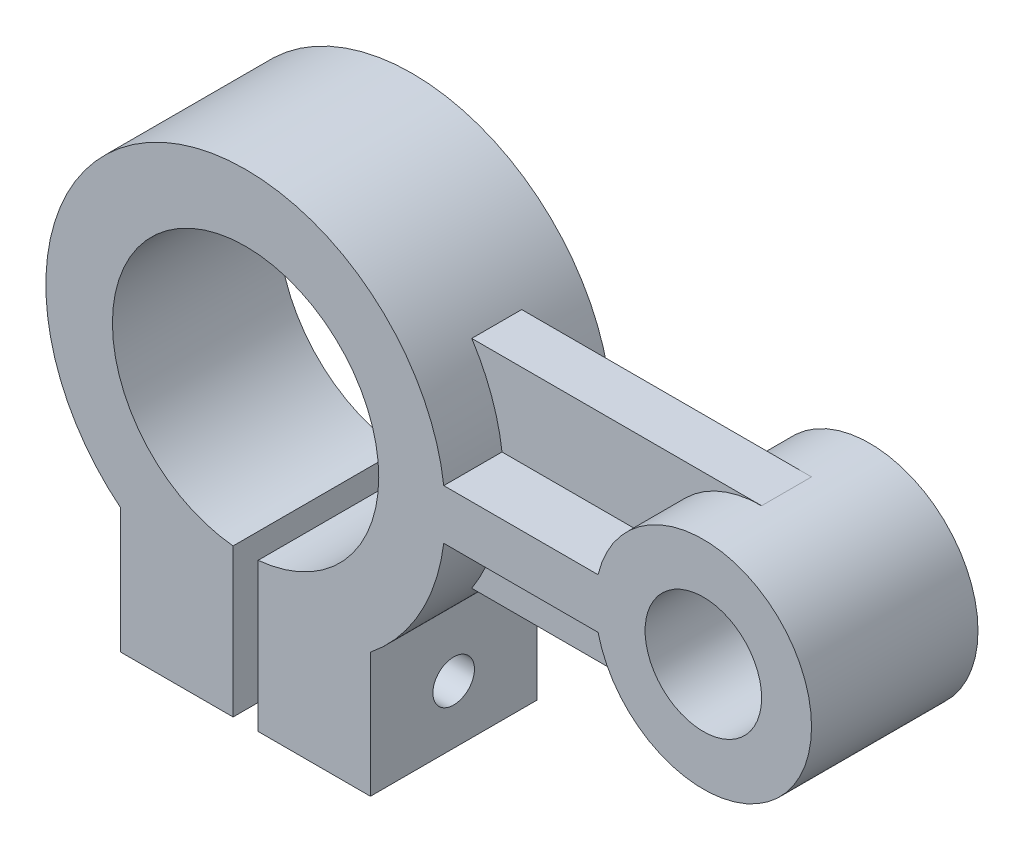
ISO-10303-21;
HEADER;
FILE_DESCRIPTION(('STEP AP214'),'2;1');
FILE_NAME('part.step','',(''),(''),'','','');
FILE_SCHEMA(('AUTOMOTIVE_DESIGN { 1 0 10303 214 1 1 1 1 }'));
ENDSEC;
DATA;
#1=APPLICATION_CONTEXT('core data for automotive mechanical design processes');
#2=APPLICATION_PROTOCOL_DEFINITION('international standard','automotive_design',2000,#1);
#3=PRODUCT_CONTEXT('',#1,'mechanical');
#4=PRODUCT('Part','Part','',(#3));
#5=PRODUCT_RELATED_PRODUCT_CATEGORY('part','',(#4));
#6=PRODUCT_DEFINITION_FORMATION('','',#4);
#7=PRODUCT_DEFINITION_CONTEXT('part definition',#1,'design');
#8=PRODUCT_DEFINITION('design','',#6,#7);
#9=PRODUCT_DEFINITION_SHAPE('','',#8);
#10=(LENGTH_UNIT() NAMED_UNIT(*) SI_UNIT(.MILLI.,.METRE.));
#11=(NAMED_UNIT(*) PLANE_ANGLE_UNIT() SI_UNIT($,.RADIAN.));
#12=(NAMED_UNIT(*) SI_UNIT($,.STERADIAN.) SOLID_ANGLE_UNIT());
#13=UNCERTAINTY_MEASURE_WITH_UNIT(LENGTH_MEASURE(1.E-05),#10,'distance_accuracy_value','');
#14=(GEOMETRIC_REPRESENTATION_CONTEXT(3) GLOBAL_UNCERTAINTY_ASSIGNED_CONTEXT((#13)) GLOBAL_UNIT_ASSIGNED_CONTEXT((#10,
#11,#12)) REPRESENTATION_CONTEXT('',''));
#15=CARTESIAN_POINT('',(0.,0.,0.));
#16=DIRECTION('',(0.,0.,1.));
#17=DIRECTION('',(1.,0.,0.));
#18=AXIS2_PLACEMENT_3D('',#15,#16,#17);
#19=CARTESIAN_POINT('',(30.,-67.4699879903904,-20.));
#20=DIRECTION('',(0.,-1.,0.));
#21=DIRECTION('',(1.,0.,0.));
#22=AXIS2_PLACEMENT_3D('',#19,#20,#21);
#23=PLANE('',#22);
#24=DIRECTION('',(0.,0.,1.));
#25=VECTOR('',#24,1.);
#26=CARTESIAN_POINT('',(-3.,-67.4699879903904,-20.));
#27=LINE('',#26,#25);
#28=CARTESIAN_POINT('',(-3.,-67.4699879903904,-20.));
#29=VERTEX_POINT('',#28);
#30=CARTESIAN_POINT('',(-3.,-67.4699879903904,20.));
#31=VERTEX_POINT('',#30);
#32=EDGE_CURVE('E179',#29,#31,#27,.T.);
#33=ORIENTED_EDGE('',*,*,#32,.T.);
#34=DIRECTION('',(1.,0.,0.));
#35=VECTOR('',#34,1.);
#36=CARTESIAN_POINT('',(30.,-67.4699879903904,20.));
#37=LINE('',#36,#35);
#38=CARTESIAN_POINT('',(-30.,-67.4699879903904,20.));
#39=VERTEX_POINT('',#38);
#40=EDGE_CURVE('E217',#39,#31,#37,.T.);
#41=ORIENTED_EDGE('',*,*,#40,.F.);
#42=DIRECTION('',(0.,0.,1.));
#43=VECTOR('',#42,1.);
#44=CARTESIAN_POINT('',(-30.,-67.4699879903904,-20.));
#45=LINE('',#44,#43);
#46=CARTESIAN_POINT('',(-30.,-67.4699879903904,-20.));
#47=VERTEX_POINT('',#46);
#48=EDGE_CURVE('E202',#47,#39,#45,.T.);
#49=ORIENTED_EDGE('',*,*,#48,.F.);
#50=DIRECTION('',(1.,0.,0.));
#51=VECTOR('',#50,1.);
#52=CARTESIAN_POINT('',(30.,-67.4699879903904,-20.));
#53=LINE('',#52,#51);
#54=EDGE_CURVE('E197',#47,#29,#53,.T.);
#55=ORIENTED_EDGE('',*,*,#54,.T.);
#56=EDGE_LOOP('',(#33,#41,#49,#55));
#57=FACE_BOUND('',#56,.T.);
#58=ADVANCED_FACE('F44',(#57),#23,.T.);
#59=CARTESIAN_POINT('',(0.,0.,20.));
#60=DIRECTION('',(0.,0.,-1.));
#61=DIRECTION('',(-1.,0.,0.));
#62=AXIS2_PLACEMENT_3D('',#59,#60,#61);
#63=CYLINDRICAL_SURFACE('',#62,48.);
#64=CARTESIAN_POINT('',(0.,0.,20.));
#65=DIRECTION('',(0.,0.,1.));
#66=DIRECTION('',(1.,0.,0.));
#67=AXIS2_PLACEMENT_3D('',#64,#65,#66);
#68=CIRCLE('',#67,48.);
#69=CARTESIAN_POINT('',(30.,-37.4699879903904,20.));
#70=VERTEX_POINT('',#69);
#71=CARTESIAN_POINT('',(47.6235235991626,-6.,20.));
#72=VERTEX_POINT('',#71);
#73=EDGE_CURVE('E324',#70,#72,#68,.T.);
#74=ORIENTED_EDGE('',*,*,#73,.F.);
#75=DIRECTION('',(0.,0.,1.));
#76=VECTOR('',#75,1.);
#77=CARTESIAN_POINT('',(30.,-37.4699879903904,-20.));
#78=LINE('',#77,#76);
#79=CARTESIAN_POINT('',(30.,-37.4699879903904,-20.));
#80=VERTEX_POINT('',#79);
#81=EDGE_CURVE('E221',#80,#70,#78,.T.);
#82=ORIENTED_EDGE('',*,*,#81,.F.);
#83=CARTESIAN_POINT('',(0.,0.,-20.));
#84=DIRECTION('',(0.,0.,1.));
#85=DIRECTION('',(1.,0.,0.));
#86=AXIS2_PLACEMENT_3D('',#83,#84,#85);
#87=CIRCLE('',#86,48.);
#88=CARTESIAN_POINT('',(47.6235235991626,-6.,-20.));
#89=VERTEX_POINT('',#88);
#90=EDGE_CURVE('E320',#80,#89,#87,.T.);
#91=ORIENTED_EDGE('',*,*,#90,.T.);
#92=DIRECTION('',(0.,0.,-1.));
#93=VECTOR('',#92,1.);
#94=CARTESIAN_POINT('',(47.6235235991626,-6.,20.));
#95=LINE('',#94,#93);
#96=CARTESIAN_POINT('',(47.6235235991626,-6.,-6.));
#97=VERTEX_POINT('',#96);
#98=EDGE_CURVE('E309',#89,#97,#95,.F.);
#99=ORIENTED_EDGE('',*,*,#98,.T.);
#100=CARTESIAN_POINT('',(0.,0.,-6.));
#101=DIRECTION('',(0.,0.,-1.));
#102=DIRECTION('',(-1.,0.,0.));
#103=AXIS2_PLACEMENT_3D('',#100,#101,#102);
#104=CIRCLE('',#103,48.);
#105=CARTESIAN_POINT('',(40.348482003664,-26.,-6.));
#106=VERTEX_POINT('',#105);
#107=EDGE_CURVE('E259',#97,#106,#104,.T.);
#108=ORIENTED_EDGE('',*,*,#107,.T.);
#109=DIRECTION('',(0.,0.,-1.));
#110=VECTOR('',#109,1.);
#111=CARTESIAN_POINT('',(40.348482003664,-26.,20.));
#112=LINE('',#111,#110);
#113=CARTESIAN_POINT('',(40.348482003664,-26.,6.));
#114=VERTEX_POINT('',#113);
#115=EDGE_CURVE('E261',#114,#106,#112,.T.);
#116=ORIENTED_EDGE('',*,*,#115,.F.);
#117=CARTESIAN_POINT('',(0.,0.,6.));
#118=DIRECTION('',(0.,0.,-1.));
#119=DIRECTION('',(-1.,0.,0.));
#120=AXIS2_PLACEMENT_3D('',#117,#118,#119);
#121=CIRCLE('',#120,48.);
#122=CARTESIAN_POINT('',(47.6235235991626,-6.,6.));
#123=VERTEX_POINT('',#122);
#124=EDGE_CURVE('E260',#123,#114,#121,.T.);
#125=ORIENTED_EDGE('',*,*,#124,.F.);
#126=EDGE_CURVE('E306',#123,#72,#95,.F.);
#127=ORIENTED_EDGE('',*,*,#126,.T.);
#128=EDGE_LOOP('',(#74,#82,#91,#99,#108,#116,#125,#127));
#129=FACE_BOUND('',#128,.T.);
#130=ADVANCED_FACE('F347',(#129),#63,.T.);
#131=CARTESIAN_POINT('',(47.6235235991626,6.,-20.));
#132=VERTEX_POINT('',#131);
#133=CARTESIAN_POINT('',(-30.,-37.4699879903904,-20.));
#134=VERTEX_POINT('',#133);
#135=EDGE_CURVE('E321',#132,#134,#87,.T.);
#136=ORIENTED_EDGE('',*,*,#135,.T.);
#137=DIRECTION('',(0.,0.,1.));
#138=VECTOR('',#137,1.);
#139=CARTESIAN_POINT('',(-30.,-37.4699879903904,-20.));
#140=LINE('',#139,#138);
#141=CARTESIAN_POINT('',(-30.,-37.4699879903904,20.));
#142=VERTEX_POINT('',#141);
#143=EDGE_CURVE('E207',#134,#142,#140,.T.);
#144=ORIENTED_EDGE('',*,*,#143,.T.);
#145=CARTESIAN_POINT('',(47.6235235991626,6.,20.));
#146=VERTEX_POINT('',#145);
#147=EDGE_CURVE('E319',#146,#142,#68,.T.);
#148=ORIENTED_EDGE('',*,*,#147,.F.);
#149=DIRECTION('',(0.,0.,-1.));
#150=VECTOR('',#149,1.);
#151=CARTESIAN_POINT('',(47.6235235991626,6.,20.));
#152=LINE('',#151,#150);
#153=CARTESIAN_POINT('',(47.6235235991626,6.,6.));
#154=VERTEX_POINT('',#153);
#155=EDGE_CURVE('E313',#146,#154,#152,.T.);
#156=ORIENTED_EDGE('',*,*,#155,.T.);
#157=CARTESIAN_POINT('',(-1.94289029309402E-13,0.,6.));
#158=DIRECTION('',(0.,0.,-1.));
#159=DIRECTION('',(-1.,0.,0.));
#160=AXIS2_PLACEMENT_3D('',#157,#158,#159);
#161=CIRCLE('',#160,48.0000000000002);
#162=CARTESIAN_POINT('',(40.348482003664,26.,6.));
#163=VERTEX_POINT('',#162);
#164=EDGE_CURVE('E272',#163,#154,#161,.T.);
#165=ORIENTED_EDGE('',*,*,#164,.F.);
#166=DIRECTION('',(0.,0.,-1.));
#167=VECTOR('',#166,1.);
#168=CARTESIAN_POINT('',(40.348482003664,26.,6.));
#169=LINE('',#168,#167);
#170=CARTESIAN_POINT('',(40.348482003664,26.,-6.));
#171=VERTEX_POINT('',#170);
#172=EDGE_CURVE('E273',#163,#171,#169,.T.);
#173=ORIENTED_EDGE('',*,*,#172,.T.);
#174=CARTESIAN_POINT('',(-1.94289029309402E-13,0.,-6.));
#175=DIRECTION('',(0.,0.,-1.));
#176=DIRECTION('',(-1.,0.,0.));
#177=AXIS2_PLACEMENT_3D('',#174,#175,#176);
#178=CIRCLE('',#177,48.0000000000002);
#179=CARTESIAN_POINT('',(47.6235235991626,6.,-6.));
#180=VERTEX_POINT('',#179);
#181=EDGE_CURVE('E277',#171,#180,#178,.T.);
#182=ORIENTED_EDGE('',*,*,#181,.T.);
#183=EDGE_CURVE('E312',#180,#132,#152,.T.);
#184=ORIENTED_EDGE('',*,*,#183,.T.);
#185=EDGE_LOOP('',(#136,#144,#148,#156,#165,#173,#182,#184));
#186=FACE_BOUND('',#185,.T.);
#187=ADVANCED_FACE('F50',(#186),#63,.T.);
#188=CARTESIAN_POINT('',(110.,0.,20.));
#189=DIRECTION('',(0.,0.,-1.));
#190=DIRECTION('',(-1.,0.,0.));
#191=AXIS2_PLACEMENT_3D('',#188,#189,#190);
#192=CYLINDRICAL_SURFACE('',#191,26.);
#193=CARTESIAN_POINT('',(110.,0.,6.));
#194=DIRECTION('',(0.,0.,-1.));
#195=DIRECTION('',(-1.,0.,0.));
#196=AXIS2_PLACEMENT_3D('',#193,#194,#195);
#197=CIRCLE('',#196,26.);
#198=CARTESIAN_POINT('',(110.,-26.,6.));
#199=VERTEX_POINT('',#198);
#200=CARTESIAN_POINT('',(84.7017787186529,-6.,6.));
#201=VERTEX_POINT('',#200);
#202=EDGE_CURVE('E240',#199,#201,#197,.T.);
#203=ORIENTED_EDGE('',*,*,#202,.F.);
#204=DIRECTION('',(0.,0.,-1.));
#205=VECTOR('',#204,1.);
#206=CARTESIAN_POINT('',(110.,-26.,6.));
#207=LINE('',#206,#205);
#208=CARTESIAN_POINT('',(110.,-26.,-6.));
#209=VERTEX_POINT('',#208);
#210=EDGE_CURVE('E250',#199,#209,#207,.T.);
#211=ORIENTED_EDGE('',*,*,#210,.T.);
#212=CARTESIAN_POINT('',(110.,0.,-6.));
#213=DIRECTION('',(0.,0.,-1.));
#214=DIRECTION('',(-1.,0.,0.));
#215=AXIS2_PLACEMENT_3D('',#212,#213,#214);
#216=CIRCLE('',#215,26.);
#217=CARTESIAN_POINT('',(84.7017787186529,-6.,-6.));
#218=VERTEX_POINT('',#217);
#219=EDGE_CURVE('E247',#209,#218,#216,.T.);
#220=ORIENTED_EDGE('',*,*,#219,.T.);
#221=DIRECTION('',(0.,0.,-1.));
#222=VECTOR('',#221,1.);
#223=CARTESIAN_POINT('',(84.7017787186529,-6.,20.));
#224=LINE('',#223,#222);
#225=CARTESIAN_POINT('',(84.7017787186529,-6.,-20.));
#226=VERTEX_POINT('',#225);
#227=EDGE_CURVE('E11',#226,#218,#224,.F.);
#228=ORIENTED_EDGE('',*,*,#227,.F.);
#229=CARTESIAN_POINT('',(110.,0.,-20.));
#230=DIRECTION('',(0.,0.,1.));
#231=DIRECTION('',(1.,0.,0.));
#232=AXIS2_PLACEMENT_3D('',#229,#230,#231);
#233=CIRCLE('',#232,26.);
#234=CARTESIAN_POINT('',(84.7017787186529,6.,-20.));
#235=VERTEX_POINT('',#234);
#236=EDGE_CURVE('E288',#226,#235,#233,.T.);
#237=ORIENTED_EDGE('',*,*,#236,.T.);
#238=DIRECTION('',(0.,0.,-1.));
#239=VECTOR('',#238,1.);
#240=CARTESIAN_POINT('',(84.7017787186529,6.,20.));
#241=LINE('',#240,#239);
#242=CARTESIAN_POINT('',(84.7017787186529,6.,-6.));
#243=VERTEX_POINT('',#242);
#244=EDGE_CURVE('E291',#243,#235,#241,.T.);
#245=ORIENTED_EDGE('',*,*,#244,.F.);
#246=CARTESIAN_POINT('',(110.,0.,-6.));
#247=DIRECTION('',(0.,0.,-1.));
#248=DIRECTION('',(-1.,0.,0.));
#249=AXIS2_PLACEMENT_3D('',#246,#247,#248);
#250=CIRCLE('',#249,26.);
#251=CARTESIAN_POINT('',(110.,26.,-6.));
#252=VERTEX_POINT('',#251);
#253=EDGE_CURVE('E263',#243,#252,#250,.T.);
#254=ORIENTED_EDGE('',*,*,#253,.T.);
#255=DIRECTION('',(0.,0.,-1.));
#256=VECTOR('',#255,1.);
#257=CARTESIAN_POINT('',(110.,26.,6.));
#258=LINE('',#257,#256);
#259=CARTESIAN_POINT('',(110.,26.,6.));
#260=VERTEX_POINT('',#259);
#261=EDGE_CURVE('E287',#260,#252,#258,.T.);
#262=ORIENTED_EDGE('',*,*,#261,.F.);
#263=CARTESIAN_POINT('',(110.,0.,6.));
#264=DIRECTION('',(0.,0.,-1.));
#265=DIRECTION('',(-1.,0.,0.));
#266=AXIS2_PLACEMENT_3D('',#263,#264,#265);
#267=CIRCLE('',#266,26.);
#268=CARTESIAN_POINT('',(84.7017787186529,6.,6.));
#269=VERTEX_POINT('',#268);
#270=EDGE_CURVE('E265',#269,#260,#267,.T.);
#271=ORIENTED_EDGE('',*,*,#270,.F.);
#272=CARTESIAN_POINT('',(84.7017787186529,6.,20.));
#273=VERTEX_POINT('',#272);
#274=EDGE_CURVE('E298',#273,#269,#241,.T.);
#275=ORIENTED_EDGE('',*,*,#274,.F.);
#276=CARTESIAN_POINT('',(110.,0.,20.));
#277=DIRECTION('',(0.,0.,1.));
#278=DIRECTION('',(1.,0.,0.));
#279=AXIS2_PLACEMENT_3D('',#276,#277,#278);
#280=CIRCLE('',#279,26.);
#281=CARTESIAN_POINT('',(84.7017787186529,-6.,20.));
#282=VERTEX_POINT('',#281);
#283=EDGE_CURVE('E290',#282,#273,#280,.T.);
#284=ORIENTED_EDGE('',*,*,#283,.F.);
#285=EDGE_CURVE('E53',#201,#282,#224,.F.);
#286=ORIENTED_EDGE('',*,*,#285,.F.);
#287=EDGE_LOOP('',(#203,#211,#220,#228,#237,#245,#254,#262,#271,#275,#284,#286));
#288=FACE_BOUND('',#287,.T.);
#289=ADVANCED_FACE('F401',(#288),#192,.T.);
#290=CARTESIAN_POINT('',(86.7905481658508,-6.,-20.));
#291=DIRECTION('',(0.,-1.,0.));
#292=DIRECTION('',(0.,0.,-1.));
#293=AXIS2_PLACEMENT_3D('',#290,#291,#292);
#294=PLANE('',#293);
#295=ORIENTED_EDGE('',*,*,#126,.F.);
#296=DIRECTION('',(-1.,0.,0.));
#297=VECTOR('',#296,1.);
#298=CARTESIAN_POINT('',(84.7017787186529,-6.,6.));
#299=LINE('',#298,#297);
#300=EDGE_CURVE('E239',#201,#123,#299,.T.);
#301=ORIENTED_EDGE('',*,*,#300,.F.);
#302=ORIENTED_EDGE('',*,*,#285,.T.);
#303=DIRECTION('',(1.,0.,0.));
#304=VECTOR('',#303,1.);
#305=CARTESIAN_POINT('',(86.7905481658508,-6.,20.));
#306=LINE('',#305,#304);
#307=EDGE_CURVE('E299',#72,#282,#306,.T.);
#308=ORIENTED_EDGE('',*,*,#307,.F.);
#309=EDGE_LOOP('',(#295,#301,#302,#308));
#310=FACE_BOUND('',#309,.T.);
#311=ADVANCED_FACE('F418',(#310),#294,.T.);
#312=CARTESIAN_POINT('',(48.,6.,-20.));
#313=DIRECTION('',(0.,1.,0.));
#314=DIRECTION('',(0.,0.,1.));
#315=AXIS2_PLACEMENT_3D('',#312,#313,#314);
#316=PLANE('',#315);
#317=ORIENTED_EDGE('',*,*,#274,.T.);
#318=DIRECTION('',(1.,0.,0.));
#319=VECTOR('',#318,1.);
#320=CARTESIAN_POINT('',(47.6235235991626,6.,6.));
#321=LINE('',#320,#319);
#322=EDGE_CURVE('E271',#154,#269,#321,.T.);
#323=ORIENTED_EDGE('',*,*,#322,.F.);
#324=ORIENTED_EDGE('',*,*,#155,.F.);
#325=DIRECTION('',(-1.,0.,0.));
#326=VECTOR('',#325,1.);
#327=CARTESIAN_POINT('',(48.,6.,20.));
#328=LINE('',#327,#326);
#329=EDGE_CURVE('E302',#273,#146,#328,.T.);
#330=ORIENTED_EDGE('',*,*,#329,.F.);
#331=EDGE_LOOP('',(#317,#323,#324,#330));
#332=FACE_BOUND('',#331,.T.);
#333=ADVANCED_FACE('F424',(#332),#316,.T.);
#334=DIRECTION('',(1.,0.,0.));
#335=VECTOR('',#334,1.);
#336=CARTESIAN_POINT('',(47.6235235991626,6.,-6.));
#337=LINE('',#336,#335);
#338=EDGE_CURVE('E268',#180,#243,#337,.T.);
#339=ORIENTED_EDGE('',*,*,#338,.T.);
#340=ORIENTED_EDGE('',*,*,#244,.T.);
#341=DIRECTION('',(-1.,0.,0.));
#342=VECTOR('',#341,1.);
#343=CARTESIAN_POINT('',(44.,6.,-20.));
#344=LINE('',#343,#342);
#345=EDGE_CURVE('E297',#235,#132,#344,.T.);
#346=ORIENTED_EDGE('',*,*,#345,.T.);
#347=ORIENTED_EDGE('',*,*,#183,.F.);
#348=EDGE_LOOP('',(#339,#340,#346,#347));
#349=FACE_BOUND('',#348,.T.);
#350=ADVANCED_FACE('F440',(#349),#316,.T.);
#351=DIRECTION('',(-1.,0.,0.));
#352=VECTOR('',#351,1.);
#353=CARTESIAN_POINT('',(84.7017787186529,-6.,-6.));
#354=LINE('',#353,#352);
#355=EDGE_CURVE('E252',#218,#97,#354,.T.);
#356=ORIENTED_EDGE('',*,*,#355,.T.);
#357=ORIENTED_EDGE('',*,*,#98,.F.);
#358=DIRECTION('',(1.,0.,0.));
#359=VECTOR('',#358,1.);
#360=CARTESIAN_POINT('',(86.7905481658508,-6.,-20.));
#361=LINE('',#360,#359);
#362=EDGE_CURVE('E303',#89,#226,#361,.T.);
#363=ORIENTED_EDGE('',*,*,#362,.T.);
#364=ORIENTED_EDGE('',*,*,#227,.T.);
#365=EDGE_LOOP('',(#356,#357,#363,#364));
#366=FACE_BOUND('',#365,.T.);
#367=ADVANCED_FACE('F406',(#366),#294,.T.);
#368=CARTESIAN_POINT('',(0.,0.,20.));
#369=DIRECTION('',(0.,0.,1.));
#370=DIRECTION('',(1.,0.,0.));
#371=AXIS2_PLACEMENT_3D('',#368,#369,#370);
#372=PLANE('',#371);
#373=DIRECTION('',(0.,-1.,0.));
#374=VECTOR('',#373,1.);
#375=CARTESIAN_POINT('',(-3.,-25.3660503355501,20.));
#376=LINE('',#375,#374);
#377=CARTESIAN_POINT('',(-3.,-31.859064644148,20.));
#378=VERTEX_POINT('',#377);
#379=EDGE_CURVE('E70',#378,#31,#376,.T.);
#380=ORIENTED_EDGE('',*,*,#379,.F.);
#381=CARTESIAN_POINT('',(0.,0.,20.));
#382=DIRECTION('',(0.,0.,1.));
#383=DIRECTION('',(1.,0.,0.));
#384=AXIS2_PLACEMENT_3D('',#381,#382,#383);
#385=CIRCLE('',#384,32.);
#386=CARTESIAN_POINT('',(3.,-31.859064644148,20.));
#387=VERTEX_POINT('',#386);
#388=EDGE_CURVE('E234',#387,#378,#385,.T.);
#389=ORIENTED_EDGE('',*,*,#388,.F.);
#390=DIRECTION('',(0.,1.,0.));
#391=VECTOR('',#390,1.);
#392=CARTESIAN_POINT('',(3.,-67.4699879903904,20.));
#393=LINE('',#392,#391);
#394=CARTESIAN_POINT('',(3.,-67.4699879903904,20.));
#395=VERTEX_POINT('',#394);
#396=EDGE_CURVE('E385',#395,#387,#393,.T.);
#397=ORIENTED_EDGE('',*,*,#396,.F.);
#398=CARTESIAN_POINT('',(30.,-67.4699879903904,20.));
#399=VERTEX_POINT('',#398);
#400=EDGE_CURVE('E212',#395,#399,#37,.T.);
#401=ORIENTED_EDGE('',*,*,#400,.T.);
#402=DIRECTION('',(0.,1.,0.));
#403=VECTOR('',#402,1.);
#404=CARTESIAN_POINT('',(30.,-37.4699879903904,20.));
#405=LINE('',#404,#403);
#406=EDGE_CURVE('E218',#399,#70,#405,.T.);
#407=ORIENTED_EDGE('',*,*,#406,.T.);
#408=ORIENTED_EDGE('',*,*,#73,.T.);
#409=ORIENTED_EDGE('',*,*,#307,.T.);
#410=ORIENTED_EDGE('',*,*,#283,.T.);
#411=ORIENTED_EDGE('',*,*,#329,.T.);
#412=ORIENTED_EDGE('',*,*,#147,.T.);
#413=DIRECTION('',(0.,-1.,0.));
#414=VECTOR('',#413,1.);
#415=CARTESIAN_POINT('',(-30.,-67.4699879903904,20.));
#416=LINE('',#415,#414);
#417=EDGE_CURVE('E211',#142,#39,#416,.T.);
#418=ORIENTED_EDGE('',*,*,#417,.T.);
#419=ORIENTED_EDGE('',*,*,#40,.T.);
#420=EDGE_LOOP('',(#380,#389,#397,#401,#407,#408,#409,#410,#411,#412,#418,#419));
#421=FACE_BOUND('',#420,.T.);
#422=CARTESIAN_POINT('',(110.,0.,20.));
#423=DIRECTION('',(0.,0.,1.));
#424=DIRECTION('',(1.,0.,0.));
#425=AXIS2_PLACEMENT_3D('',#422,#423,#424);
#426=CIRCLE('',#425,14.);
#427=CARTESIAN_POINT('',(124.,0.,20.));
#428=VERTEX_POINT('',#427);
#429=EDGE_CURVE('E223',#428,#428,#426,.T.);
#430=ORIENTED_EDGE('',*,*,#429,.F.);
#431=EDGE_LOOP('',(#430));
#432=FACE_BOUND('',#431,.T.);
#433=ADVANCED_FACE('F377',(#421,#432),#372,.T.);
#434=CARTESIAN_POINT('',(0.,0.,-20.));
#435=DIRECTION('',(0.,0.,1.));
#436=DIRECTION('',(1.,0.,0.));
#437=AXIS2_PLACEMENT_3D('',#434,#435,#436);
#438=PLANE('',#437);
#439=CARTESIAN_POINT('',(110.,0.,-20.));
#440=DIRECTION('',(0.,0.,1.));
#441=DIRECTION('',(1.,0.,0.));
#442=AXIS2_PLACEMENT_3D('',#439,#440,#441);
#443=CIRCLE('',#442,14.);
#444=CARTESIAN_POINT('',(124.,0.,-20.));
#445=VERTEX_POINT('',#444);
#446=EDGE_CURVE('E231',#445,#445,#443,.T.);
#447=ORIENTED_EDGE('',*,*,#446,.T.);
#448=EDGE_LOOP('',(#447));
#449=FACE_BOUND('',#448,.T.);
#450=CARTESIAN_POINT('',(0.,0.,-20.));
#451=DIRECTION('',(0.,0.,1.));
#452=DIRECTION('',(1.,0.,0.));
#453=AXIS2_PLACEMENT_3D('',#450,#451,#452);
#454=CIRCLE('',#453,32.);
#455=CARTESIAN_POINT('',(3.,-31.859064644148,-20.));
#456=VERTEX_POINT('',#455);
#457=CARTESIAN_POINT('',(-3.,-31.859064644148,-20.));
#458=VERTEX_POINT('',#457);
#459=EDGE_CURVE('E200',#456,#458,#454,.T.);
#460=ORIENTED_EDGE('',*,*,#459,.T.);
#461=DIRECTION('',(0.,-1.,0.));
#462=VECTOR('',#461,1.);
#463=CARTESIAN_POINT('',(-3.,-25.3660503355501,-20.));
#464=LINE('',#463,#462);
#465=EDGE_CURVE('E182',#458,#29,#464,.T.);
#466=ORIENTED_EDGE('',*,*,#465,.T.);
#467=ORIENTED_EDGE('',*,*,#54,.F.);
#468=DIRECTION('',(0.,-1.,0.));
#469=VECTOR('',#468,1.);
#470=CARTESIAN_POINT('',(-30.,-67.4699879903904,-20.));
#471=LINE('',#470,#469);
#472=EDGE_CURVE('E206',#134,#47,#471,.T.);
#473=ORIENTED_EDGE('',*,*,#472,.F.);
#474=ORIENTED_EDGE('',*,*,#135,.F.);
#475=ORIENTED_EDGE('',*,*,#345,.F.);
#476=ORIENTED_EDGE('',*,*,#236,.F.);
#477=ORIENTED_EDGE('',*,*,#362,.F.);
#478=ORIENTED_EDGE('',*,*,#90,.F.);
#479=DIRECTION('',(0.,1.,0.));
#480=VECTOR('',#479,1.);
#481=CARTESIAN_POINT('',(30.,-37.4699879903904,-20.));
#482=LINE('',#481,#480);
#483=CARTESIAN_POINT('',(30.,-67.4699879903904,-20.));
#484=VERTEX_POINT('',#483);
#485=EDGE_CURVE('E204',#484,#80,#482,.T.);
#486=ORIENTED_EDGE('',*,*,#485,.F.);
#487=CARTESIAN_POINT('',(3.,-67.4699879903904,-20.));
#488=VERTEX_POINT('',#487);
#489=EDGE_CURVE('E203',#488,#484,#53,.T.);
#490=ORIENTED_EDGE('',*,*,#489,.F.);
#491=DIRECTION('',(0.,1.,0.));
#492=VECTOR('',#491,1.);
#493=CARTESIAN_POINT('',(3.,-67.4699879903904,-20.));
#494=LINE('',#493,#492);
#495=EDGE_CURVE('E61',#488,#456,#494,.T.);
#496=ORIENTED_EDGE('',*,*,#495,.T.);
#497=EDGE_LOOP('',(#460,#466,#467,#473,#474,#475,#476,#477,#478,#486,#490,#496));
#498=FACE_BOUND('',#497,.T.);
#499=ADVANCED_FACE('F192',(#449,#498),#438,.F.);
#500=CARTESIAN_POINT('',(110.,26.,6.));
#501=DIRECTION('',(0.,-1.,0.));
#502=DIRECTION('',(0.,0.,-1.));
#503=AXIS2_PLACEMENT_3D('',#500,#501,#502);
#504=PLANE('',#503);
#505=DIRECTION('',(-1.,0.,0.));
#506=VECTOR('',#505,1.);
#507=CARTESIAN_POINT('',(110.,26.,-6.));
#508=LINE('',#507,#506);
#509=EDGE_CURVE('E280',#252,#171,#508,.T.);
#510=ORIENTED_EDGE('',*,*,#509,.T.);
#511=ORIENTED_EDGE('',*,*,#172,.F.);
#512=DIRECTION('',(-1.,0.,0.));
#513=VECTOR('',#512,1.);
#514=CARTESIAN_POINT('',(110.,26.,6.));
#515=LINE('',#514,#513);
#516=EDGE_CURVE('E269',#260,#163,#515,.T.);
#517=ORIENTED_EDGE('',*,*,#516,.F.);
#518=ORIENTED_EDGE('',*,*,#261,.T.);
#519=EDGE_LOOP('',(#510,#511,#517,#518));
#520=FACE_BOUND('',#519,.T.);
#521=ADVANCED_FACE('F435',(#520),#504,.F.);
#522=CARTESIAN_POINT('',(110.,0.,6.));
#523=DIRECTION('',(0.,0.,-1.));
#524=DIRECTION('',(-1.,0.,0.));
#525=AXIS2_PLACEMENT_3D('',#522,#523,#524);
#526=PLANE('',#525);
#527=ORIENTED_EDGE('',*,*,#270,.T.);
#528=ORIENTED_EDGE('',*,*,#516,.T.);
#529=ORIENTED_EDGE('',*,*,#164,.T.);
#530=ORIENTED_EDGE('',*,*,#322,.T.);
#531=EDGE_LOOP('',(#527,#528,#529,#530));
#532=FACE_BOUND('',#531,.T.);
#533=ADVANCED_FACE('F429',(#532),#526,.F.);
#534=CARTESIAN_POINT('',(110.,0.,-6.));
#535=DIRECTION('',(0.,0.,-1.));
#536=DIRECTION('',(-1.,0.,0.));
#537=AXIS2_PLACEMENT_3D('',#534,#535,#536);
#538=PLANE('',#537);
#539=ORIENTED_EDGE('',*,*,#253,.F.);
#540=ORIENTED_EDGE('',*,*,#338,.F.);
#541=ORIENTED_EDGE('',*,*,#181,.F.);
#542=ORIENTED_EDGE('',*,*,#509,.F.);
#543=EDGE_LOOP('',(#539,#540,#541,#542));
#544=FACE_BOUND('',#543,.T.);
#545=ADVANCED_FACE('F436',(#544),#538,.T.);
#546=CARTESIAN_POINT('',(110.,-26.,6.));
#547=DIRECTION('',(0.,1.,0.));
#548=DIRECTION('',(0.,0.,1.));
#549=AXIS2_PLACEMENT_3D('',#546,#547,#548);
#550=PLANE('',#549);
#551=DIRECTION('',(1.,0.,0.));
#552=VECTOR('',#551,1.);
#553=CARTESIAN_POINT('',(110.,-26.,6.));
#554=LINE('',#553,#552);
#555=EDGE_CURVE('E242',#114,#199,#554,.T.);
#556=ORIENTED_EDGE('',*,*,#555,.F.);
#557=ORIENTED_EDGE('',*,*,#115,.T.);
#558=DIRECTION('',(1.,0.,0.));
#559=VECTOR('',#558,1.);
#560=CARTESIAN_POINT('',(110.,-26.,-6.));
#561=LINE('',#560,#559);
#562=EDGE_CURVE('E241',#106,#209,#561,.T.);
#563=ORIENTED_EDGE('',*,*,#562,.T.);
#564=ORIENTED_EDGE('',*,*,#210,.F.);
#565=EDGE_LOOP('',(#556,#557,#563,#564));
#566=FACE_BOUND('',#565,.T.);
#567=ADVANCED_FACE('F413',(#566),#550,.F.);
#568=CARTESIAN_POINT('',(110.,0.,6.));
#569=DIRECTION('',(0.,0.,-1.));
#570=DIRECTION('',(-1.,0.,0.));
#571=AXIS2_PLACEMENT_3D('',#568,#569,#570);
#572=PLANE('',#571);
#573=ORIENTED_EDGE('',*,*,#300,.T.);
#574=ORIENTED_EDGE('',*,*,#124,.T.);
#575=ORIENTED_EDGE('',*,*,#555,.T.);
#576=ORIENTED_EDGE('',*,*,#202,.T.);
#577=EDGE_LOOP('',(#573,#574,#575,#576));
#578=FACE_BOUND('',#577,.T.);
#579=ADVANCED_FACE('F416',(#578),#572,.F.);
#580=CARTESIAN_POINT('',(110.,0.,-6.));
#581=DIRECTION('',(0.,0.,-1.));
#582=DIRECTION('',(-1.,0.,0.));
#583=AXIS2_PLACEMENT_3D('',#580,#581,#582);
#584=PLANE('',#583);
#585=ORIENTED_EDGE('',*,*,#107,.F.);
#586=ORIENTED_EDGE('',*,*,#355,.F.);
#587=ORIENTED_EDGE('',*,*,#219,.F.);
#588=ORIENTED_EDGE('',*,*,#562,.F.);
#589=EDGE_LOOP('',(#585,#586,#587,#588));
#590=FACE_BOUND('',#589,.T.);
#591=ADVANCED_FACE('F341',(#590),#584,.T.);
#592=CARTESIAN_POINT('',(0.,0.,-193.));
#593=DIRECTION('',(0.,0.,1.));
#594=DIRECTION('',(1.,0.,0.));
#595=AXIS2_PLACEMENT_3D('',#592,#593,#594);
#596=CYLINDRICAL_SURFACE('',#595,32.);
#597=ORIENTED_EDGE('',*,*,#388,.T.);
#598=DIRECTION('',(0.,0.,1.));
#599=VECTOR('',#598,1.);
#600=CARTESIAN_POINT('',(-3.,-31.859064644148,-193.));
#601=LINE('',#600,#599);
#602=EDGE_CURVE('E216',#378,#458,#601,.F.);
#603=ORIENTED_EDGE('',*,*,#602,.T.);
#604=ORIENTED_EDGE('',*,*,#459,.F.);
#605=DIRECTION('',(0.,0.,1.));
#606=VECTOR('',#605,1.);
#607=CARTESIAN_POINT('',(3.,-31.859064644148,-193.));
#608=LINE('',#607,#606);
#609=EDGE_CURVE('E186',#456,#387,#608,.T.);
#610=ORIENTED_EDGE('',*,*,#609,.T.);
#611=EDGE_LOOP('',(#597,#603,#604,#610));
#612=FACE_BOUND('',#611,.T.);
#613=ADVANCED_FACE('F332',(#612),#596,.F.);
#614=CARTESIAN_POINT('',(110.,0.,-193.));
#615=DIRECTION('',(0.,0.,1.));
#616=DIRECTION('',(1.,0.,0.));
#617=AXIS2_PLACEMENT_3D('',#614,#615,#616);
#618=CYLINDRICAL_SURFACE('',#617,14.);
#619=ORIENTED_EDGE('',*,*,#429,.T.);
#620=EDGE_LOOP('',(#619));
#621=FACE_BOUND('',#620,.T.);
#622=ORIENTED_EDGE('',*,*,#446,.F.);
#623=EDGE_LOOP('',(#622));
#624=FACE_BOUND('',#623,.T.);
#625=ADVANCED_FACE('F328',(#621,#624),#618,.F.);
#626=CARTESIAN_POINT('',(30.,-37.4699879903904,-20.));
#627=DIRECTION('',(1.,0.,0.));
#628=DIRECTION('',(0.,1.,0.));
#629=AXIS2_PLACEMENT_3D('',#626,#627,#628);
#630=PLANE('',#629);
#631=CARTESIAN_POINT('',(30.,-53.4699879903904,0.));
#632=DIRECTION('',(1.,0.,0.));
#633=DIRECTION('',(0.,1.,0.));
#634=AXIS2_PLACEMENT_3D('',#631,#632,#633);
#635=CIRCLE('',#634,5.);
#636=CARTESIAN_POINT('',(30.,-48.4699879903904,0.));
#637=VERTEX_POINT('',#636);
#638=EDGE_CURVE('E799',#637,#637,#635,.T.);
#639=ORIENTED_EDGE('',*,*,#638,.F.);
#640=EDGE_LOOP('',(#639));
#641=FACE_BOUND('',#640,.T.);
#642=ORIENTED_EDGE('',*,*,#406,.F.);
#643=DIRECTION('',(0.,0.,1.));
#644=VECTOR('',#643,1.);
#645=CARTESIAN_POINT('',(30.,-67.4699879903904,-20.));
#646=LINE('',#645,#644);
#647=EDGE_CURVE('E225',#484,#399,#646,.T.);
#648=ORIENTED_EDGE('',*,*,#647,.F.);
#649=ORIENTED_EDGE('',*,*,#485,.T.);
#650=ORIENTED_EDGE('',*,*,#81,.T.);
#651=EDGE_LOOP('',(#642,#648,#649,#650));
#652=FACE_BOUND('',#651,.T.);
#653=ADVANCED_FACE('F331',(#641,#652),#630,.T.);
#654=DIRECTION('',(0.,0.,1.));
#655=VECTOR('',#654,1.);
#656=CARTESIAN_POINT('',(3.,-67.4699879903904,-20.));
#657=LINE('',#656,#655);
#658=EDGE_CURVE('E188',#488,#395,#657,.T.);
#659=ORIENTED_EDGE('',*,*,#658,.F.);
#660=ORIENTED_EDGE('',*,*,#489,.T.);
#661=ORIENTED_EDGE('',*,*,#647,.T.);
#662=ORIENTED_EDGE('',*,*,#400,.F.);
#663=EDGE_LOOP('',(#659,#660,#661,#662));
#664=FACE_BOUND('',#663,.T.);
#665=ADVANCED_FACE('F339',(#664),#23,.T.);
#666=CARTESIAN_POINT('',(-30.,-67.4699879903904,-20.));
#667=DIRECTION('',(-1.,0.,0.));
#668=DIRECTION('',(0.,0.,1.));
#669=AXIS2_PLACEMENT_3D('',#666,#667,#668);
#670=PLANE('',#669);
#671=CARTESIAN_POINT('',(-30.,-53.4699879903904,0.));
#672=DIRECTION('',(-1.,0.,0.));
#673=DIRECTION('',(0.,0.,1.));
#674=AXIS2_PLACEMENT_3D('',#671,#672,#673);
#675=CIRCLE('',#674,5.);
#676=CARTESIAN_POINT('',(-30.,-48.4699879903904,0.));
#677=VERTEX_POINT('',#676);
#678=EDGE_CURVE('E381',#677,#677,#675,.T.);
#679=ORIENTED_EDGE('',*,*,#678,.F.);
#680=EDGE_LOOP('',(#679));
#681=FACE_BOUND('',#680,.T.);
#682=ORIENTED_EDGE('',*,*,#417,.F.);
#683=ORIENTED_EDGE('',*,*,#143,.F.);
#684=ORIENTED_EDGE('',*,*,#472,.T.);
#685=ORIENTED_EDGE('',*,*,#48,.T.);
#686=EDGE_LOOP('',(#682,#683,#684,#685));
#687=FACE_BOUND('',#686,.T.);
#688=ADVANCED_FACE('F353',(#681,#687),#670,.T.);
#689=CARTESIAN_POINT('',(3.,-67.4699879903904,-20.));
#690=DIRECTION('',(1.,0.,0.));
#691=DIRECTION('',(0.,0.,-1.));
#692=AXIS2_PLACEMENT_3D('',#689,#690,#691);
#693=PLANE('',#692);
#694=CARTESIAN_POINT('',(3.,-53.4699879903904,0.));
#695=DIRECTION('',(1.,0.,0.));
#696=DIRECTION('',(0.,0.,-1.));
#697=AXIS2_PLACEMENT_3D('',#694,#695,#696);
#698=CIRCLE('',#697,5.);
#699=CARTESIAN_POINT('',(3.,-48.4699879903904,0.));
#700=VERTEX_POINT('',#699);
#701=EDGE_CURVE('E390',#700,#700,#698,.T.);
#702=ORIENTED_EDGE('',*,*,#701,.T.);
#703=EDGE_LOOP('',(#702));
#704=FACE_BOUND('',#703,.T.);
#705=ORIENTED_EDGE('',*,*,#495,.F.);
#706=ORIENTED_EDGE('',*,*,#658,.T.);
#707=ORIENTED_EDGE('',*,*,#396,.T.);
#708=ORIENTED_EDGE('',*,*,#609,.F.);
#709=EDGE_LOOP('',(#705,#706,#707,#708));
#710=FACE_BOUND('',#709,.T.);
#711=ADVANCED_FACE('F360',(#704,#710),#693,.F.);
#712=CARTESIAN_POINT('',(-3.,-25.3660503355501,-20.));
#713=DIRECTION('',(-1.,0.,0.));
#714=DIRECTION('',(0.,-1.,0.));
#715=AXIS2_PLACEMENT_3D('',#712,#713,#714);
#716=PLANE('',#715);
#717=CARTESIAN_POINT('',(-3.,-53.4699879903904,0.));
#718=DIRECTION('',(-1.,0.,0.));
#719=DIRECTION('',(0.,-1.,0.));
#720=AXIS2_PLACEMENT_3D('',#717,#718,#719);
#721=CIRCLE('',#720,5.);
#722=CARTESIAN_POINT('',(-3.,-48.4699879903904,0.));
#723=VERTEX_POINT('',#722);
#724=EDGE_CURVE('E47',#723,#723,#721,.T.);
#725=ORIENTED_EDGE('',*,*,#724,.T.);
#726=EDGE_LOOP('',(#725));
#727=FACE_BOUND('',#726,.T.);
#728=ORIENTED_EDGE('',*,*,#379,.T.);
#729=ORIENTED_EDGE('',*,*,#32,.F.);
#730=ORIENTED_EDGE('',*,*,#465,.F.);
#731=ORIENTED_EDGE('',*,*,#602,.F.);
#732=EDGE_LOOP('',(#728,#729,#730,#731));
#733=FACE_BOUND('',#732,.T.);
#734=ADVANCED_FACE('F185',(#727,#733),#716,.F.);
#735=CARTESIAN_POINT('',(-75.0000000000001,-53.4699879903904,0.));
#736=DIRECTION('',(1.,0.,0.));
#737=DIRECTION('',(0.,1.,0.));
#738=AXIS2_PLACEMENT_3D('',#735,#736,#737);
#739=CYLINDRICAL_SURFACE('',#738,5.);
#740=CARTESIAN_POINT('',(-30.,-48.4699879903904,0.));
#741=CARTESIAN_POINT('',(-29.71875,-48.4699879903904,0.));
#742=CARTESIAN_POINT('',(-29.4375,-48.4699879903904,0.));
#743=CARTESIAN_POINT('',(-28.875,-48.4699879903904,0.));
#744=CARTESIAN_POINT('',(-28.59375,-48.4699879903904,0.));
#745=CARTESIAN_POINT('',(-28.03125,-48.4699879903904,0.));
#746=CARTESIAN_POINT('',(-27.75,-48.4699879903904,0.));
#747=CARTESIAN_POINT('',(-27.1875,-48.4699879903904,0.));
#748=CARTESIAN_POINT('',(-26.90625,-48.4699879903904,0.));
#749=CARTESIAN_POINT('',(-26.34375,-48.4699879903904,0.));
#750=CARTESIAN_POINT('',(-26.0625,-48.4699879903904,0.));
#751=CARTESIAN_POINT('',(-25.5,-48.4699879903904,0.));
#752=CARTESIAN_POINT('',(-25.21875,-48.4699879903904,0.));
#753=CARTESIAN_POINT('',(-24.65625,-48.4699879903904,0.));
#754=CARTESIAN_POINT('',(-24.375,-48.4699879903904,0.));
#755=CARTESIAN_POINT('',(-23.8125,-48.4699879903904,0.));
#756=CARTESIAN_POINT('',(-23.53125,-48.4699879903904,0.));
#757=CARTESIAN_POINT('',(-22.96875,-48.4699879903904,0.));
#758=CARTESIAN_POINT('',(-22.6875,-48.4699879903904,0.));
#759=CARTESIAN_POINT('',(-22.125,-48.4699879903904,0.));
#760=CARTESIAN_POINT('',(-21.84375,-48.4699879903904,0.));
#761=CARTESIAN_POINT('',(-21.28125,-48.4699879903904,0.));
#762=CARTESIAN_POINT('',(-21.,-48.4699879903904,0.));
#763=CARTESIAN_POINT('',(-20.4375,-48.4699879903904,0.));
#764=CARTESIAN_POINT('',(-20.15625,-48.4699879903904,0.));
#765=CARTESIAN_POINT('',(-19.59375,-48.4699879903904,0.));
#766=CARTESIAN_POINT('',(-19.3125,-48.4699879903904,0.));
#767=CARTESIAN_POINT('',(-18.75,-48.4699879903904,0.));
#768=CARTESIAN_POINT('',(-18.46875,-48.4699879903904,0.));
#769=CARTESIAN_POINT('',(-17.90625,-48.4699879903904,0.));
#770=CARTESIAN_POINT('',(-17.625,-48.4699879903904,0.));
#771=CARTESIAN_POINT('',(-17.0625,-48.4699879903904,0.));
#772=CARTESIAN_POINT('',(-16.78125,-48.4699879903904,0.));
#773=CARTESIAN_POINT('',(-16.21875,-48.4699879903904,0.));
#774=CARTESIAN_POINT('',(-15.9375,-48.4699879903904,0.));
#775=CARTESIAN_POINT('',(-15.375,-48.4699879903904,0.));
#776=CARTESIAN_POINT('',(-15.09375,-48.4699879903904,0.));
#777=CARTESIAN_POINT('',(-14.53125,-48.4699879903904,0.));
#778=CARTESIAN_POINT('',(-14.25,-48.4699879903904,0.));
#779=CARTESIAN_POINT('',(-13.6875,-48.4699879903904,0.));
#780=CARTESIAN_POINT('',(-13.40625,-48.4699879903904,0.));
#781=CARTESIAN_POINT('',(-12.84375,-48.4699879903904,0.));
#782=CARTESIAN_POINT('',(-12.5625,-48.4699879903904,0.));
#783=CARTESIAN_POINT('',(-12.,-48.4699879903904,0.));
#784=CARTESIAN_POINT('',(-11.71875,-48.4699879903904,0.));
#785=CARTESIAN_POINT('',(-11.15625,-48.4699879903904,0.));
#786=CARTESIAN_POINT('',(-10.875,-48.4699879903904,0.));
#787=CARTESIAN_POINT('',(-10.3125,-48.4699879903904,0.));
#788=CARTESIAN_POINT('',(-10.03125,-48.4699879903904,0.));
#789=CARTESIAN_POINT('',(-9.46875000000001,-48.4699879903904,0.));
#790=CARTESIAN_POINT('',(-9.18750000000001,-48.4699879903904,0.));
#791=CARTESIAN_POINT('',(-8.625,-48.4699879903904,0.));
#792=CARTESIAN_POINT('',(-8.34375,-48.4699879903904,0.));
#793=CARTESIAN_POINT('',(-7.78125,-48.4699879903904,0.));
#794=CARTESIAN_POINT('',(-7.5,-48.4699879903904,0.));
#795=CARTESIAN_POINT('',(-6.9375,-48.4699879903904,0.));
#796=CARTESIAN_POINT('',(-6.65625,-48.4699879903904,0.));
#797=CARTESIAN_POINT('',(-6.09375,-48.4699879903904,0.));
#798=CARTESIAN_POINT('',(-5.8125,-48.4699879903904,0.));
#799=CARTESIAN_POINT('',(-5.25,-48.4699879903904,0.));
#800=CARTESIAN_POINT('',(-4.96875000000001,-48.4699879903904,0.));
#801=CARTESIAN_POINT('',(-4.40625000000001,-48.4699879903904,0.));
#802=CARTESIAN_POINT('',(-4.12500000000001,-48.4699879903904,0.));
#803=CARTESIAN_POINT('',(-3.56250000000001,-48.4699879903904,0.));
#804=CARTESIAN_POINT('',(-3.28125,-48.4699879903904,0.));
#805=CARTESIAN_POINT('',(-3.,-48.4699879903904,0.));
#806=B_SPLINE_CURVE_WITH_KNOTS('',3,(#740,#741,#742,#743,#744,#745,#746,#747,#748,#749,#750,
#751,#752,#753,#754,#755,#756,#757,#758,#759,#760,#761,#762,#763,#764,#765,#766,#767,#768,#769,
#770,#771,#772,#773,#774,#775,#776,#777,#778,#779,#780,#781,#782,#783,#784,#785,#786,#787,#788,
#789,#790,#791,#792,#793,#794,#795,#796,#797,#798,#799,#800,#801,#802,#803,#804,#805),
.UNSPECIFIED.,.F.,.F.,(4,2,2,2,2,2,2,2,2,2,2,2,2,2,2,2,2,2,2,2,2,2,2,2,2,2,2,2,2,2,2,2,4),(0.,
0.843749999999997,1.6875,2.53125,3.375,4.21875,5.0625,5.90625,6.75,7.59375,8.4375,9.28125,
10.125,10.96875,11.8125,12.65625,13.5,14.34375,15.1875,16.03125,16.875,17.71875,18.5625,
19.40625,20.25,21.09375,21.9375,22.78125,23.625,24.46875,25.3125,26.15625,27.),.UNSPECIFIED.);
#807=EDGE_CURVE('BSEAM521',#677,#723,#806,.T.);
#808=ORIENTED_EDGE('',*,*,#678,.T.);
#809=ORIENTED_EDGE('',*,*,#724,.F.);
#810=ORIENTED_EDGE('',*,*,#807,.T.);
#811=ORIENTED_EDGE('',*,*,#807,.F.);
#812=EDGE_LOOP('',(#808,#810,#809,#811));
#813=FACE_BOUND('',#812,.T.);
#814=ADVANCED_FACE('F521',(#813),#739,.F.);
#815=CARTESIAN_POINT('',(30.,-48.4699879903904,0.));
#816=CARTESIAN_POINT('',(29.71875,-48.4699879903904,0.));
#817=CARTESIAN_POINT('',(29.4375,-48.4699879903904,0.));
#818=CARTESIAN_POINT('',(28.875,-48.4699879903904,0.));
#819=CARTESIAN_POINT('',(28.59375,-48.4699879903904,0.));
#820=CARTESIAN_POINT('',(28.03125,-48.4699879903904,0.));
#821=CARTESIAN_POINT('',(27.75,-48.4699879903904,0.));
#822=CARTESIAN_POINT('',(27.1875,-48.4699879903904,0.));
#823=CARTESIAN_POINT('',(26.90625,-48.4699879903904,0.));
#824=CARTESIAN_POINT('',(26.34375,-48.4699879903904,0.));
#825=CARTESIAN_POINT('',(26.0625,-48.4699879903904,0.));
#826=CARTESIAN_POINT('',(25.5,-48.4699879903904,0.));
#827=CARTESIAN_POINT('',(25.21875,-48.4699879903904,0.));
#828=CARTESIAN_POINT('',(24.65625,-48.4699879903904,0.));
#829=CARTESIAN_POINT('',(24.375,-48.4699879903904,0.));
#830=CARTESIAN_POINT('',(23.8125,-48.4699879903904,0.));
#831=CARTESIAN_POINT('',(23.53125,-48.4699879903904,0.));
#832=CARTESIAN_POINT('',(22.96875,-48.4699879903904,0.));
#833=CARTESIAN_POINT('',(22.6875,-48.4699879903904,0.));
#834=CARTESIAN_POINT('',(22.125,-48.4699879903904,0.));
#835=CARTESIAN_POINT('',(21.84375,-48.4699879903904,0.));
#836=CARTESIAN_POINT('',(21.28125,-48.4699879903904,0.));
#837=CARTESIAN_POINT('',(21.,-48.4699879903904,0.));
#838=CARTESIAN_POINT('',(20.4375,-48.4699879903904,0.));
#839=CARTESIAN_POINT('',(20.15625,-48.4699879903904,0.));
#840=CARTESIAN_POINT('',(19.59375,-48.4699879903904,0.));
#841=CARTESIAN_POINT('',(19.3125,-48.4699879903904,0.));
#842=CARTESIAN_POINT('',(18.75,-48.4699879903904,0.));
#843=CARTESIAN_POINT('',(18.46875,-48.4699879903904,0.));
#844=CARTESIAN_POINT('',(17.90625,-48.4699879903904,0.));
#845=CARTESIAN_POINT('',(17.625,-48.4699879903904,0.));
#846=CARTESIAN_POINT('',(17.0625,-48.4699879903904,0.));
#847=CARTESIAN_POINT('',(16.78125,-48.4699879903904,0.));
#848=CARTESIAN_POINT('',(16.21875,-48.4699879903904,0.));
#849=CARTESIAN_POINT('',(15.9375,-48.4699879903904,0.));
#850=CARTESIAN_POINT('',(15.375,-48.4699879903904,0.));
#851=CARTESIAN_POINT('',(15.09375,-48.4699879903904,0.));
#852=CARTESIAN_POINT('',(14.53125,-48.4699879903904,0.));
#853=CARTESIAN_POINT('',(14.25,-48.4699879903904,0.));
#854=CARTESIAN_POINT('',(13.6875,-48.4699879903904,0.));
#855=CARTESIAN_POINT('',(13.40625,-48.4699879903904,0.));
#856=CARTESIAN_POINT('',(12.84375,-48.4699879903904,0.));
#857=CARTESIAN_POINT('',(12.5625,-48.4699879903904,0.));
#858=CARTESIAN_POINT('',(12.,-48.4699879903904,0.));
#859=CARTESIAN_POINT('',(11.71875,-48.4699879903904,0.));
#860=CARTESIAN_POINT('',(11.15625,-48.4699879903904,0.));
#861=CARTESIAN_POINT('',(10.875,-48.4699879903904,0.));
#862=CARTESIAN_POINT('',(10.3125,-48.4699879903904,0.));
#863=CARTESIAN_POINT('',(10.03125,-48.4699879903904,0.));
#864=CARTESIAN_POINT('',(9.46875000000001,-48.4699879903904,0.));
#865=CARTESIAN_POINT('',(9.18750000000001,-48.4699879903904,0.));
#866=CARTESIAN_POINT('',(8.625,-48.4699879903904,0.));
#867=CARTESIAN_POINT('',(8.34375,-48.4699879903904,0.));
#868=CARTESIAN_POINT('',(7.78125,-48.4699879903904,0.));
#869=CARTESIAN_POINT('',(7.5,-48.4699879903904,0.));
#870=CARTESIAN_POINT('',(6.9375,-48.4699879903904,0.));
#871=CARTESIAN_POINT('',(6.65625,-48.4699879903904,0.));
#872=CARTESIAN_POINT('',(6.09375,-48.4699879903904,0.));
#873=CARTESIAN_POINT('',(5.8125,-48.4699879903904,0.));
#874=CARTESIAN_POINT('',(5.25,-48.4699879903904,0.));
#875=CARTESIAN_POINT('',(4.96875000000001,-48.4699879903904,0.));
#876=CARTESIAN_POINT('',(4.40625000000001,-48.4699879903904,0.));
#877=CARTESIAN_POINT('',(4.12500000000001,-48.4699879903904,0.));
#878=CARTESIAN_POINT('',(3.56250000000001,-48.4699879903904,0.));
#879=CARTESIAN_POINT('',(3.28125,-48.4699879903904,0.));
#880=CARTESIAN_POINT('',(3.,-48.4699879903904,0.));
#881=B_SPLINE_CURVE_WITH_KNOTS('',3,(#815,#816,#817,#818,#819,#820,#821,#822,#823,#824,#825,
#826,#827,#828,#829,#830,#831,#832,#833,#834,#835,#836,#837,#838,#839,#840,#841,#842,#843,#844,
#845,#846,#847,#848,#849,#850,#851,#852,#853,#854,#855,#856,#857,#858,#859,#860,#861,#862,#863,
#864,#865,#866,#867,#868,#869,#870,#871,#872,#873,#874,#875,#876,#877,#878,#879,#880),
.UNSPECIFIED.,.F.,.F.,(4,2,2,2,2,2,2,2,2,2,2,2,2,2,2,2,2,2,2,2,2,2,2,2,2,2,2,2,2,2,2,2,4),(0.,
0.843750000000004,1.68749999999999,2.53125,3.375,4.21874999999999,5.0625,5.90625,
6.75000000000001,7.59375,8.4375,9.28124999999999,10.125,10.96875,11.8125,12.65625,13.5,14.34375,
15.1875,16.03125,16.875,17.71875,18.5625,19.40625,20.25,21.09375,21.9375,22.78125,23.625,
24.46875,25.3125,26.15625,27.),.UNSPECIFIED.);
#882=EDGE_CURVE('BSEAM532',#637,#700,#881,.T.);
#883=ORIENTED_EDGE('',*,*,#638,.T.);
#884=ORIENTED_EDGE('',*,*,#701,.F.);
#885=ORIENTED_EDGE('',*,*,#882,.T.);
#886=ORIENTED_EDGE('',*,*,#882,.F.);
#887=EDGE_LOOP('',(#883,#885,#884,#886));
#888=FACE_BOUND('',#887,.T.);
#889=ADVANCED_FACE('F532',(#888),#739,.F.);
#890=CLOSED_SHELL('',(#58,#130,#187,#289,#311,#333,#350,#367,#433,#499,#521,#533,#545,#567,#579,
#591,#613,#625,#653,#665,#688,#711,#734,#814,#889));
#891=MANIFOLD_SOLID_BREP('B2',#890);
#892=ADVANCED_BREP_SHAPE_REPRESENTATION('',(#18,#891),#14);
#893=SHAPE_DEFINITION_REPRESENTATION(#9,#892);
ENDSEC;
END-ISO-10303-21;
